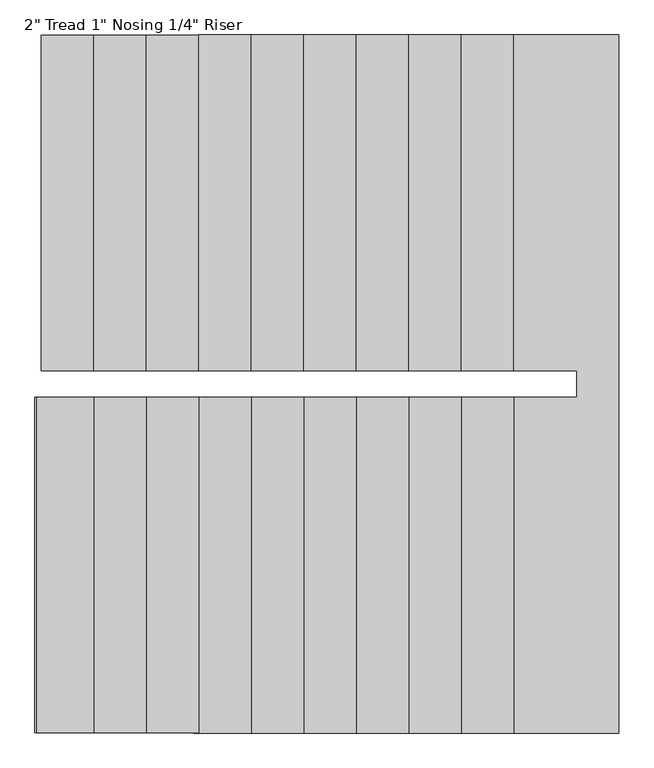
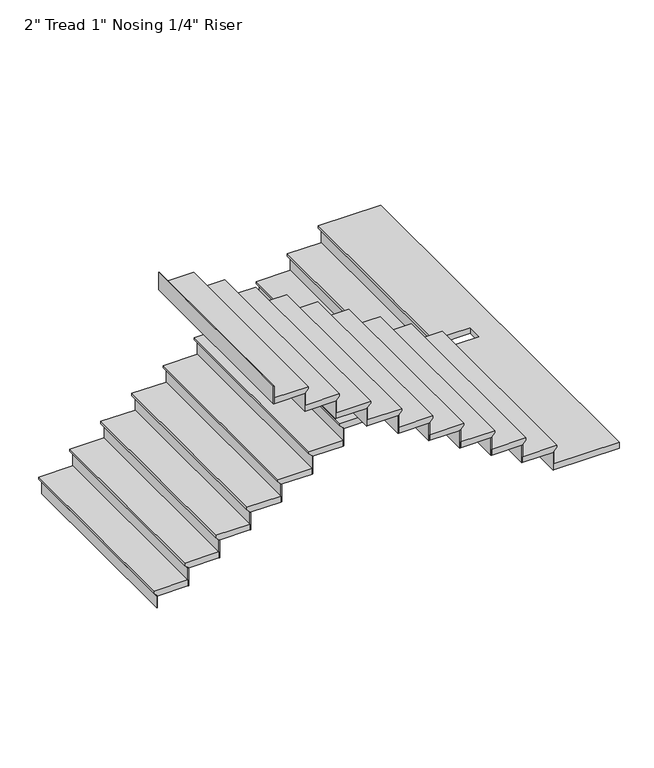
"""IFC4 building model written with IfcOpenShell, lengths in millimetres: stair flight geometry."""

from ifc_helpers import new_model, si_unit, origin, place, context, project, spatial, faceted_brep, source, transform, mapped, element, save


def stair_flight_8d4d0c3c(model_context):
    return source(origin(), model_context, "Body", "Brep", [
        faceted_brep([(-6414.1711241, 10106.9344295, 6229.35), (-6414.1711241, 10106.9344295, 6248.4), (-6414.1711241, 11732.5344295, 6248.4), (-6414.1711241, 11732.5344295, 6229.35), (-6388.7711241, 10106.9344295, 6203.95), (-6388.7711241, 11732.5344295, 6203.95), (-6134.7711241, 10106.9344295, 6248.4), (-6134.7711241, 11732.5344295, 6248.4), (-6388.7711241, 11732.5344295, 6197.6), (-6134.7711241, 11732.5344295, 6197.6), (-6134.7711241, 10106.9344295, 6197.6), (-6388.7711241, 10106.9344295, 6197.6)], [[[0, 1, 2, 3]], [[4, 0, 3, 5]], [[2, 1, 6, 7]], [[8, 9, 10, 11]], [[2, 7, 9, 8, 5, 3]], [[8, 11, 4, 5]], [[6, 1, 0, 4, 11, 10]], [[7, 6, 10, 9]]]),
        faceted_brep([(-6388.7711241, 10106.9344295, 6197.6), (-6388.7711241, 10106.9344295, 6096.0), (-6382.4211241, 10106.9344295, 6096.0), (-6382.4211241, 10106.9344295, 6197.6), (-6388.7711241, 11732.5344295, 6197.6), (-6382.4211241, 11732.5344295, 6197.6), (-6382.4211241, 11732.5344295, 6096.0), (-6388.7711241, 11732.5344295, 6096.0)], [[[0, 1, 2, 3]], [[4, 5, 6, 7]], [[1, 0, 4, 7]], [[2, 1, 7, 6]], [[3, 2, 6, 5]], [[0, 3, 5, 4]]]),
        faceted_brep([(-6134.7711241, 10106.9344295, 6350.0), (-6134.7711241, 10106.9344295, 6197.6), (-6128.4211241, 10106.9344295, 6197.6), (-6128.4211241, 10106.9344295, 6350.0), (-6134.7711241, 11732.5344295, 6350.0), (-6128.4211241, 11732.5344295, 6350.0), (-6128.4211241, 11732.5344295, 6197.6), (-6134.7711241, 11732.5344295, 6197.6)], [[[0, 1, 2, 3]], [[4, 5, 6, 7]], [[1, 0, 4, 7]], [[2, 1, 7, 6]], [[3, 2, 6, 5]], [[0, 3, 5, 4]]]),
        faceted_brep([(-6160.1711241, 11732.5344295, 6400.8), (-6160.1711241, 10106.9344295, 6400.8), (-5880.7711241, 10106.9344295, 6400.8), (-5880.7711241, 11732.5344295, 6400.8), (-6134.7711241, 11732.5344295, 6350.0), (-5880.7711241, 11732.5344295, 6350.0), (-5880.7711241, 10106.9344295, 6350.0), (-6134.7711241, 10106.9344295, 6350.0), (-6134.7711241, 11732.5344295, 6356.35), (-6160.1711241, 11732.5344295, 6381.75), (-6134.7711241, 10106.9344295, 6356.35), (-6160.1711241, 10106.9344295, 6381.75)], [[[0, 1, 2, 3]], [[4, 5, 6, 7]], [[0, 3, 5, 4, 8, 9]], [[4, 7, 10, 8]], [[2, 1, 11, 10, 7, 6]], [[3, 2, 6, 5]], [[11, 1, 0, 9]], [[10, 11, 9, 8]]]),
        faceted_brep([(-5880.7711241, 10106.9344295, 6502.4), (-5880.7711241, 10106.9344295, 6350.0), (-5874.4211241, 10106.9344295, 6350.0), (-5874.4211241, 10106.9344295, 6502.4), (-5880.7711241, 11732.5344295, 6502.4), (-5874.4211241, 11732.5344295, 6502.4), (-5874.4211241, 11732.5344295, 6350.0), (-5880.7711241, 11732.5344295, 6350.0)], [[[0, 1, 2, 3]], [[4, 5, 6, 7]], [[1, 0, 4, 7]], [[2, 1, 7, 6]], [[3, 2, 6, 5]], [[0, 3, 5, 4]]]),
        faceted_brep([(-5906.1711241, 11732.5344295, 6553.2), (-5906.1711241, 10106.9344295, 6553.2), (-5626.7711241, 10106.9344295, 6553.2), (-5626.7711241, 11732.5344295, 6553.2), (-5880.7711241, 11732.5344295, 6502.4), (-5626.7711241, 11732.5344295, 6502.4), (-5626.7711241, 10106.9344295, 6502.4), (-5880.7711241, 10106.9344295, 6502.4), (-5880.7711241, 11732.5344295, 6508.75), (-5906.1711241, 11732.5344295, 6534.15), (-5880.7711241, 10106.9344295, 6508.75), (-5906.1711241, 10106.9344295, 6534.15)], [[[0, 1, 2, 3]], [[4, 5, 6, 7]], [[0, 3, 5, 4, 8, 9]], [[4, 7, 10, 8]], [[2, 1, 11, 10, 7, 6]], [[3, 2, 6, 5]], [[11, 1, 0, 9]], [[10, 11, 9, 8]]]),
        faceted_brep([(-5626.7711241, 10106.9344295, 6654.8), (-5626.7711241, 10106.9344295, 6502.4), (-5620.4211241, 10106.9344295, 6502.4), (-5620.4211241, 10106.9344295, 6654.8), (-5626.7711241, 11732.5344295, 6654.8), (-5620.4211241, 11732.5344295, 6654.8), (-5620.4211241, 11732.5344295, 6502.4), (-5626.7711241, 11732.5344295, 6502.4)], [[[0, 1, 2, 3]], [[4, 5, 6, 7]], [[1, 0, 4, 7]], [[2, 1, 7, 6]], [[3, 2, 6, 5]], [[0, 3, 5, 4]]]),
        faceted_brep([(-5652.1711241, 11732.5344295, 6705.6), (-5652.1711241, 10106.9344295, 6705.6), (-5372.7711241, 10106.9344295, 6705.6), (-5372.7711241, 11732.5344295, 6705.6), (-5626.7711241, 11732.5344295, 6654.8), (-5372.7711241, 11732.5344295, 6654.8), (-5372.7711241, 10106.9344295, 6654.8), (-5626.7711241, 10106.9344295, 6654.8), (-5626.7711241, 11732.5344295, 6661.15), (-5652.1711241, 11732.5344295, 6686.55), (-5626.7711241, 10106.9344295, 6661.15), (-5652.1711241, 10106.9344295, 6686.55)], [[[0, 1, 2, 3]], [[4, 5, 6, 7]], [[0, 3, 5, 4, 8, 9]], [[4, 7, 10, 8]], [[2, 1, 11, 10, 7, 6]], [[3, 2, 6, 5]], [[11, 1, 0, 9]], [[10, 11, 9, 8]]]),
        faceted_brep([(-5372.7711241, 10106.9344295, 6807.2), (-5372.7711241, 10106.9344295, 6654.8), (-5366.4211241, 10106.9344295, 6654.8), (-5366.4211241, 10106.9344295, 6807.2), (-5372.7711241, 11732.5344295, 6807.2), (-5366.4211241, 11732.5344295, 6807.2), (-5366.4211241, 11732.5344295, 6654.8), (-5372.7711241, 11732.5344295, 6654.8)], [[[0, 1, 2, 3]], [[4, 5, 6, 7]], [[1, 0, 4, 7]], [[2, 1, 7, 6]], [[3, 2, 6, 5]], [[0, 3, 5, 4]]]),
        faceted_brep([(-5398.1711241, 11732.5344295, 6858.0), (-5398.1711241, 10106.9344295, 6858.0), (-5118.7711241, 10106.9344295, 6858.0), (-5118.7711241, 11732.5344295, 6858.0), (-5372.7711241, 11732.5344295, 6807.2), (-5118.7711241, 11732.5344295, 6807.2), (-5118.7711241, 10106.9344295, 6807.2), (-5372.7711241, 10106.9344295, 6807.2), (-5372.7711241, 11732.5344295, 6813.55), (-5398.1711241, 11732.5344295, 6838.95), (-5372.7711241, 10106.9344295, 6813.55), (-5398.1711241, 10106.9344295, 6838.95)], [[[0, 1, 2, 3]], [[4, 5, 6, 7]], [[0, 3, 5, 4, 8, 9]], [[4, 7, 10, 8]], [[2, 1, 11, 10, 7, 6]], [[3, 2, 6, 5]], [[11, 1, 0, 9]], [[10, 11, 9, 8]]]),
        faceted_brep([(-5118.7711241, 10106.9344295, 6959.6), (-5118.7711241, 10106.9344295, 6807.2), (-5112.4211241, 10106.9344295, 6807.2), (-5112.4211241, 10106.9344295, 6959.6), (-5118.7711241, 11732.5344295, 6959.6), (-5112.4211241, 11732.5344295, 6959.6), (-5112.4211241, 11732.5344295, 6807.2), (-5118.7711241, 11732.5344295, 6807.2)], [[[0, 1, 2, 3]], [[4, 5, 6, 7]], [[1, 0, 4, 7]], [[2, 1, 7, 6]], [[3, 2, 6, 5]], [[0, 3, 5, 4]]]),
        faceted_brep([(-5144.1711241, 11732.5344295, 7010.4), (-5144.1711241, 10106.9344295, 7010.4), (-4864.7711241, 10106.9344295, 7010.4), (-4864.7711241, 11732.5344295, 7010.4), (-5118.7711241, 11732.5344295, 6959.6), (-4864.7711241, 11732.5344295, 6959.6), (-4864.7711241, 10106.9344295, 6959.6), (-5118.7711241, 10106.9344295, 6959.6), (-5118.7711241, 11732.5344295, 6965.95), (-5144.1711241, 11732.5344295, 6991.35), (-5118.7711241, 10106.9344295, 6965.95), (-5144.1711241, 10106.9344295, 6991.35)], [[[0, 1, 2, 3]], [[4, 5, 6, 7]], [[0, 3, 5, 4, 8, 9]], [[4, 7, 10, 8]], [[2, 1, 11, 10, 7, 6]], [[3, 2, 6, 5]], [[11, 1, 0, 9]], [[10, 11, 9, 8]]]),
        faceted_brep([(-4864.7711241, 10106.9344295, 7112.0), (-4864.7711241, 10106.9344295, 6959.6), (-4858.4211241, 10106.9344295, 6959.6), (-4858.4211241, 10106.9344295, 7112.0), (-4864.7711241, 11732.5344295, 7112.0), (-4858.4211241, 11732.5344295, 7112.0), (-4858.4211241, 11732.5344295, 6959.6), (-4864.7711241, 11732.5344295, 6959.6)], [[[0, 1, 2, 3]], [[4, 5, 6, 7]], [[1, 0, 4, 7]], [[2, 1, 7, 6]], [[3, 2, 6, 5]], [[0, 3, 5, 4]]]),
        faceted_brep([(-4890.1711241, 11732.5344295, 7162.8), (-4890.1711241, 10106.9344295, 7162.8), (-4610.7711241, 10106.9344295, 7162.8), (-4610.7711241, 11732.5344295, 7162.8), (-4864.7711241, 11732.5344295, 7112.0), (-4610.7711241, 11732.5344295, 7112.0), (-4610.7711241, 10106.9344295, 7112.0), (-4864.7711241, 10106.9344295, 7112.0), (-4864.7711241, 11732.5344295, 7118.35), (-4890.1711241, 11732.5344295, 7143.75), (-4864.7711241, 10106.9344295, 7118.35), (-4890.1711241, 10106.9344295, 7143.75)], [[[0, 1, 2, 3]], [[4, 5, 6, 7]], [[0, 3, 5, 4, 8, 9]], [[4, 7, 10, 8]], [[2, 1, 11, 10, 7, 6]], [[3, 2, 6, 5]], [[11, 1, 0, 9]], [[10, 11, 9, 8]]]),
        faceted_brep([(-4610.7711241, 10106.9344295, 7264.4), (-4610.7711241, 10106.9344295, 7112.0), (-4604.4211241, 10106.9344295, 7112.0), (-4604.4211241, 10106.9344295, 7264.4), (-4610.7711241, 11732.5344295, 7264.4), (-4604.4211241, 11732.5344295, 7264.4), (-4604.4211241, 11732.5344295, 7112.0), (-4610.7711241, 11732.5344295, 7112.0)], [[[0, 1, 2, 3]], [[4, 5, 6, 7]], [[1, 0, 4, 7]], [[2, 1, 7, 6]], [[3, 2, 6, 5]], [[0, 3, 5, 4]]]),
        faceted_brep([(-4636.1711241, 11732.5344295, 7315.2), (-4636.1711241, 10106.9344295, 7315.2), (-4356.7711241, 10106.9344295, 7315.2), (-4356.7711241, 11732.5344295, 7315.2), (-4610.7711241, 11732.5344295, 7264.4), (-4356.7711241, 11732.5344295, 7264.4), (-4356.7711241, 10106.9344295, 7264.4), (-4610.7711241, 10106.9344295, 7264.4), (-4610.7711241, 11732.5344295, 7270.75), (-4636.1711241, 11732.5344295, 7296.15), (-4610.7711241, 10106.9344295, 7270.75), (-4636.1711241, 10106.9344295, 7296.15)], [[[0, 1, 2, 3]], [[4, 5, 6, 7]], [[0, 3, 5, 4, 8, 9]], [[4, 7, 10, 8]], [[2, 1, 11, 10, 7, 6]], [[3, 2, 6, 5]], [[11, 1, 0, 9]], [[10, 11, 9, 8]]]),
        faceted_brep([(-4356.7711241, 10106.9344295, 7416.8), (-4356.7711241, 10106.9344295, 7264.4), (-4350.4211241, 10106.9344295, 7264.4), (-4350.4211241, 10106.9344295, 7416.8), (-4356.7711241, 11732.5344295, 7416.8), (-4350.4211241, 11732.5344295, 7416.8), (-4350.4211241, 11732.5344295, 7264.4), (-4356.7711241, 11732.5344295, 7264.4)], [[[0, 1, 2, 3]], [[4, 5, 6, 7]], [[1, 0, 4, 7]], [[2, 1, 7, 6]], [[3, 2, 6, 5]], [[0, 3, 5, 4]]]),
        faceted_brep([(-4382.1711241, 11732.5344295, 7467.6), (-4382.1711241, 10106.9344295, 7467.6), (-4102.7711241, 10106.9344295, 7467.6), (-4102.7711241, 11732.5344295, 7467.6), (-4356.7711241, 11732.5344295, 7416.8), (-4102.7711241, 11732.5344295, 7416.8), (-4102.7711241, 10106.9344295, 7416.8), (-4356.7711241, 10106.9344295, 7416.8), (-4356.7711241, 11732.5344295, 7423.15), (-4382.1711241, 11732.5344295, 7448.55), (-4356.7711241, 10106.9344295, 7423.15), (-4382.1711241, 10106.9344295, 7448.55)], [[[0, 1, 2, 3]], [[4, 5, 6, 7]], [[0, 3, 5, 4, 8, 9]], [[4, 7, 10, 8]], [[2, 1, 11, 10, 7, 6]], [[3, 2, 6, 5]], [[11, 1, 0, 9]], [[10, 11, 9, 8]]]),
        faceted_brep([(-4102.7711241, 10106.9344295, 7569.2), (-4102.7711241, 10106.9344295, 7416.8), (-4096.4211241, 10106.9344295, 7416.8), (-4096.4211241, 10106.9344295, 7569.2), (-4102.7711241, 11732.5344295, 7569.2), (-4096.4211241, 11732.5344295, 7569.2), (-4096.4211241, 11732.5344295, 7416.8), (-4102.7711241, 11732.5344295, 7416.8)], [[[0, 1, 2, 3]], [[4, 5, 6, 7]], [[1, 0, 4, 7]], [[2, 1, 7, 6]], [[3, 2, 6, 5]], [[0, 3, 5, 4]]]),
        faceted_brep([(-4153.5711241, 8354.3344295, 7620.0), (-3620.1711241, 8354.3344295, 7620.0), (-3620.1711241, 11732.5344295, 7620.0), (-4128.1711241, 11732.5344295, 7620.0), (-4128.1711241, 10106.9344295, 7620.0), (-3823.3711241, 10106.9344295, 7620.0), (-3823.3711241, 9979.9344295, 7620.0), (-4153.5711241, 9979.9344295, 7620.0), (-3620.1711241, 8354.3344295, 7569.2), (-4153.5711241, 8354.3344295, 7569.2), (-4153.5711241, 9979.9344295, 7569.2), (-3823.3711241, 9979.9344295, 7569.2), (-3823.3711241, 10106.9344295, 7569.2), (-4102.7711241, 10106.9344295, 7569.2), (-4102.7711241, 11732.5344295, 7569.2), (-3620.1711241, 11732.5344295, 7569.2), (-4102.7711241, 11732.5344295, 7575.55), (-4128.1711241, 11732.5344295, 7600.95), (-4102.7711241, 10106.9344295, 7575.55), (-4128.1711241, 10106.9344295, 7600.95)], [[[0, 1, 2, 3, 4, 5, 6, 7]], [[8, 9, 10, 11, 12, 13, 14, 15]], [[1, 0, 9, 8]], [[2, 1, 8, 15]], [[3, 2, 15, 14, 16, 17]], [[14, 13, 18, 16]], [[5, 4, 19, 18, 13, 12]], [[6, 5, 12, 11]], [[7, 6, 11, 10]], [[0, 7, 10, 9]], [[19, 4, 3, 17]], [[18, 19, 17, 16]]]),
        faceted_brep([(-4153.5711241, 9979.9344295, 7721.6), (-4153.5711241, 9979.9344295, 7569.2), (-4159.9211241, 9979.9344295, 7569.2), (-4159.9211241, 9979.9344295, 7721.6), (-4153.5711241, 8354.3344295, 7721.6), (-4159.9211241, 8354.3344295, 7721.6), (-4159.9211241, 8354.3344295, 7569.2), (-4153.5711241, 8354.3344295, 7569.2)], [[[0, 1, 2, 3]], [[4, 5, 6, 7]], [[1, 0, 4, 7]], [[2, 1, 7, 6]], [[3, 2, 6, 5]], [[0, 3, 5, 4]]]),
        faceted_brep([(-4128.1711241, 8354.3344295, 7772.4), (-4128.1711241, 9979.9344295, 7772.4), (-4407.5711241, 9979.9344295, 7772.4), (-4407.5711241, 8354.3344295, 7772.4), (-4153.5711241, 8354.3344295, 7721.6), (-4407.5711241, 8354.3344295, 7721.6), (-4407.5711241, 9979.9344295, 7721.6), (-4153.5711241, 9979.9344295, 7721.6), (-4153.5711241, 8354.3344295, 7727.95), (-4128.1711241, 8354.3344295, 7753.35), (-4153.5711241, 9979.9344295, 7727.95), (-4128.1711241, 9979.9344295, 7753.35)], [[[0, 1, 2, 3]], [[4, 5, 6, 7]], [[0, 3, 5, 4, 8, 9]], [[4, 7, 10, 8]], [[2, 1, 11, 10, 7, 6]], [[3, 2, 6, 5]], [[11, 1, 0, 9]], [[10, 11, 9, 8]]]),
        faceted_brep([(-4407.5711241, 9979.9344295, 7874.0), (-4407.5711241, 9979.9344295, 7721.6), (-4413.9211241, 9979.9344295, 7721.6), (-4413.9211241, 9979.9344295, 7874.0), (-4407.5711241, 8354.3344295, 7874.0), (-4413.9211241, 8354.3344295, 7874.0), (-4413.9211241, 8354.3344295, 7721.6), (-4407.5711241, 8354.3344295, 7721.6)], [[[0, 1, 2, 3]], [[4, 5, 6, 7]], [[1, 0, 4, 7]], [[2, 1, 7, 6]], [[3, 2, 6, 5]], [[0, 3, 5, 4]]]),
        faceted_brep([(-4382.1711241, 8354.3344295, 7924.8), (-4382.1711241, 9979.9344295, 7924.8), (-4661.5711241, 9979.9344295, 7924.8), (-4661.5711241, 8354.3344295, 7924.8), (-4407.5711241, 8354.3344295, 7874.0), (-4661.5711241, 8354.3344295, 7874.0), (-4661.5711241, 9979.9344295, 7874.0), (-4407.5711241, 9979.9344295, 7874.0), (-4407.5711241, 8354.3344295, 7880.35), (-4382.1711241, 8354.3344295, 7905.75), (-4407.5711241, 9979.9344295, 7880.35), (-4382.1711241, 9979.9344295, 7905.75)], [[[0, 1, 2, 3]], [[4, 5, 6, 7]], [[0, 3, 5, 4, 8, 9]], [[4, 7, 10, 8]], [[2, 1, 11, 10, 7, 6]], [[3, 2, 6, 5]], [[11, 1, 0, 9]], [[10, 11, 9, 8]]]),
        faceted_brep([(-4661.5711241, 9979.9344295, 8026.4), (-4661.5711241, 9979.9344295, 7874.0), (-4667.9211241, 9979.9344295, 7874.0), (-4667.9211241, 9979.9344295, 8026.4), (-4661.5711241, 8354.3344295, 8026.4), (-4667.9211241, 8354.3344295, 8026.4), (-4667.9211241, 8354.3344295, 7874.0), (-4661.5711241, 8354.3344295, 7874.0)], [[[0, 1, 2, 3]], [[4, 5, 6, 7]], [[1, 0, 4, 7]], [[2, 1, 7, 6]], [[3, 2, 6, 5]], [[0, 3, 5, 4]]]),
        faceted_brep([(-4636.1711241, 8354.3344295, 8077.2), (-4636.1711241, 9979.9344295, 8077.2), (-4915.5711241, 9979.9344295, 8077.2), (-4915.5711241, 8354.3344295, 8077.2), (-4661.5711241, 8354.3344295, 8026.4), (-4915.5711241, 8354.3344295, 8026.4), (-4915.5711241, 9979.9344295, 8026.4), (-4661.5711241, 9979.9344295, 8026.4), (-4661.5711241, 8354.3344295, 8032.75), (-4636.1711241, 8354.3344295, 8058.15), (-4661.5711241, 9979.9344295, 8032.75), (-4636.1711241, 9979.9344295, 8058.15)], [[[0, 1, 2, 3]], [[4, 5, 6, 7]], [[0, 3, 5, 4, 8, 9]], [[4, 7, 10, 8]], [[2, 1, 11, 10, 7, 6]], [[3, 2, 6, 5]], [[11, 1, 0, 9]], [[10, 11, 9, 8]]]),
        faceted_brep([(-4915.5711241, 9979.9344295, 8178.8), (-4915.5711241, 9979.9344295, 8026.4), (-4921.9211241, 9979.9344295, 8026.4), (-4921.9211241, 9979.9344295, 8178.8), (-4915.5711241, 8354.3344295, 8178.8), (-4921.9211241, 8354.3344295, 8178.8), (-4921.9211241, 8354.3344295, 8026.4), (-4915.5711241, 8354.3344295, 8026.4)], [[[0, 1, 2, 3]], [[4, 5, 6, 7]], [[1, 0, 4, 7]], [[2, 1, 7, 6]], [[3, 2, 6, 5]], [[0, 3, 5, 4]]]),
        faceted_brep([(-4890.1711241, 8354.3344295, 8229.6), (-4890.1711241, 9979.9344295, 8229.6), (-5169.5711241, 9979.9344295, 8229.6), (-5169.5711241, 8354.3344295, 8229.6), (-4915.5711241, 8354.3344295, 8178.8), (-5169.5711241, 8354.3344295, 8178.8), (-5169.5711241, 9979.9344295, 8178.8), (-4915.5711241, 9979.9344295, 8178.8), (-4915.5711241, 8354.3344295, 8185.15), (-4890.1711241, 8354.3344295, 8210.55), (-4915.5711241, 9979.9344295, 8185.15), (-4890.1711241, 9979.9344295, 8210.55)], [[[0, 1, 2, 3]], [[4, 5, 6, 7]], [[0, 3, 5, 4, 8, 9]], [[4, 7, 10, 8]], [[2, 1, 11, 10, 7, 6]], [[3, 2, 6, 5]], [[11, 1, 0, 9]], [[10, 11, 9, 8]]]),
        faceted_brep([(-5169.5711241, 9979.9344295, 8331.2), (-5169.5711241, 9979.9344295, 8178.8), (-5175.9211241, 9979.9344295, 8178.8), (-5175.9211241, 9979.9344295, 8331.2), (-5169.5711241, 8354.3344295, 8331.2), (-5175.9211241, 8354.3344295, 8331.2), (-5175.9211241, 8354.3344295, 8178.8), (-5169.5711241, 8354.3344295, 8178.8)], [[[0, 1, 2, 3]], [[4, 5, 6, 7]], [[1, 0, 4, 7]], [[2, 1, 7, 6]], [[3, 2, 6, 5]], [[0, 3, 5, 4]]]),
        faceted_brep([(-5144.1711241, 8354.3344295, 8382.0), (-5144.1711241, 9979.9344295, 8382.0), (-5423.5711241, 9979.9344295, 8382.0), (-5423.5711241, 8354.3344295, 8382.0), (-5169.5711241, 8354.3344295, 8331.2), (-5423.5711241, 8354.3344295, 8331.2), (-5423.5711241, 9979.9344295, 8331.2), (-5169.5711241, 9979.9344295, 8331.2), (-5169.5711241, 8354.3344295, 8337.55), (-5144.1711241, 8354.3344295, 8362.95), (-5169.5711241, 9979.9344295, 8337.55), (-5144.1711241, 9979.9344295, 8362.95)], [[[0, 1, 2, 3]], [[4, 5, 6, 7]], [[0, 3, 5, 4, 8, 9]], [[4, 7, 10, 8]], [[2, 1, 11, 10, 7, 6]], [[3, 2, 6, 5]], [[11, 1, 0, 9]], [[10, 11, 9, 8]]]),
        faceted_brep([(-5423.5711241, 9979.9344295, 8483.6), (-5423.5711241, 9979.9344295, 8331.2), (-5429.9211241, 9979.9344295, 8331.2), (-5429.9211241, 9979.9344295, 8483.6), (-5423.5711241, 8354.3344295, 8483.6), (-5429.9211241, 8354.3344295, 8483.6), (-5429.9211241, 8354.3344295, 8331.2), (-5423.5711241, 8354.3344295, 8331.2)], [[[0, 1, 2, 3]], [[4, 5, 6, 7]], [[1, 0, 4, 7]], [[2, 1, 7, 6]], [[3, 2, 6, 5]], [[0, 3, 5, 4]]]),
        faceted_brep([(-5398.1711241, 8354.3344295, 8534.4), (-5398.1711241, 9979.9344295, 8534.4), (-5677.5711241, 9979.9344295, 8534.4), (-5677.5711241, 8354.3344295, 8534.4), (-5423.5711241, 8354.3344295, 8483.6), (-5677.5711241, 8354.3344295, 8483.6), (-5677.5711241, 9979.9344295, 8483.6), (-5423.5711241, 9979.9344295, 8483.6), (-5423.5711241, 8354.3344295, 8489.95), (-5398.1711241, 8354.3344295, 8515.35), (-5423.5711241, 9979.9344295, 8489.95), (-5398.1711241, 9979.9344295, 8515.35)], [[[0, 1, 2, 3]], [[4, 5, 6, 7]], [[0, 3, 5, 4, 8, 9]], [[4, 7, 10, 8]], [[2, 1, 11, 10, 7, 6]], [[3, 2, 6, 5]], [[11, 1, 0, 9]], [[10, 11, 9, 8]]]),
        faceted_brep([(-5677.5711241, 9979.9344295, 8636.0), (-5677.5711241, 9979.9344295, 8483.6), (-5683.9211241, 9979.9344295, 8483.6), (-5683.9211241, 9979.9344295, 8636.0), (-5677.5711241, 8354.3344295, 8636.0), (-5683.9211241, 8354.3344295, 8636.0), (-5683.9211241, 8354.3344295, 8483.6), (-5677.5711241, 8354.3344295, 8483.6)], [[[0, 1, 2, 3]], [[4, 5, 6, 7]], [[1, 0, 4, 7]], [[2, 1, 7, 6]], [[3, 2, 6, 5]], [[0, 3, 5, 4]]]),
        faceted_brep([(-5652.1711241, 8354.3344295, 8686.8), (-5652.1711241, 9979.9344295, 8686.8), (-5931.5711241, 9979.9344295, 8686.8), (-5931.5711241, 8354.3344295, 8686.8), (-5677.5711241, 8354.3344295, 8636.0), (-5931.5711241, 8354.3344295, 8636.0), (-5931.5711241, 9979.9344295, 8636.0), (-5677.5711241, 9979.9344295, 8636.0), (-5677.5711241, 8354.3344295, 8642.35), (-5652.1711241, 8354.3344295, 8667.75), (-5677.5711241, 9979.9344295, 8642.35), (-5652.1711241, 9979.9344295, 8667.75)], [[[0, 1, 2, 3]], [[4, 5, 6, 7]], [[0, 3, 5, 4, 8, 9]], [[4, 7, 10, 8]], [[2, 1, 11, 10, 7, 6]], [[3, 2, 6, 5]], [[11, 1, 0, 9]], [[10, 11, 9, 8]]]),
        faceted_brep([(-5931.5711241, 9979.9344295, 8788.4), (-5931.5711241, 9979.9344295, 8636.0), (-5937.9211241, 9979.9344295, 8636.0), (-5937.9211241, 9979.9344295, 8788.4), (-5931.5711241, 8354.3344295, 8788.4), (-5937.9211241, 8354.3344295, 8788.4), (-5937.9211241, 8354.3344295, 8636.0), (-5931.5711241, 8354.3344295, 8636.0)], [[[0, 1, 2, 3]], [[4, 5, 6, 7]], [[1, 0, 4, 7]], [[2, 1, 7, 6]], [[3, 2, 6, 5]], [[0, 3, 5, 4]]]),
        faceted_brep([(-5906.1711241, 8354.3344295, 8839.2), (-5906.1711241, 9979.9344295, 8839.2), (-6185.5711241, 9979.9344295, 8839.2), (-6185.5711241, 8354.3344295, 8839.2), (-5931.5711241, 8354.3344295, 8788.4), (-6185.5711241, 8354.3344295, 8788.4), (-6185.5711241, 9979.9344295, 8788.4), (-5931.5711241, 9979.9344295, 8788.4), (-5931.5711241, 8354.3344295, 8794.75), (-5906.1711241, 8354.3344295, 8820.15), (-5931.5711241, 9979.9344295, 8794.75), (-5906.1711241, 9979.9344295, 8820.15)], [[[0, 1, 2, 3]], [[4, 5, 6, 7]], [[0, 3, 5, 4, 8, 9]], [[4, 7, 10, 8]], [[2, 1, 11, 10, 7, 6]], [[3, 2, 6, 5]], [[11, 1, 0, 9]], [[10, 11, 9, 8]]]),
        faceted_brep([(-6185.5711241, 9979.9344295, 8940.8), (-6185.5711241, 9979.9344295, 8788.4), (-6191.9211241, 9979.9344295, 8788.4), (-6191.9211241, 9979.9344295, 8940.8), (-6185.5711241, 8354.3344295, 8940.8), (-6191.9211241, 8354.3344295, 8940.8), (-6191.9211241, 8354.3344295, 8788.4), (-6185.5711241, 8354.3344295, 8788.4)], [[[0, 1, 2, 3]], [[4, 5, 6, 7]], [[1, 0, 4, 7]], [[2, 1, 7, 6]], [[3, 2, 6, 5]], [[0, 3, 5, 4]]]),
        faceted_brep([(-6439.5711241, 9979.9344295, 9093.2), (-6439.5711241, 9979.9344295, 8940.8), (-6445.9211241, 9979.9344295, 8940.8), (-6445.9211241, 9979.9344295, 9093.2), (-6439.5711241, 8354.3344295, 9093.2), (-6445.9211241, 8354.3344295, 9093.2), (-6445.9211241, 8354.3344295, 8940.8), (-6439.5711241, 8354.3344295, 8940.8)], [[[0, 1, 2, 3]], [[4, 5, 6, 7]], [[1, 0, 4, 7]], [[2, 1, 7, 6]], [[3, 2, 6, 5]], [[0, 3, 5, 4]]]),
        faceted_brep([(-6160.1711241, 8354.3344295, 8991.6), (-6160.1711241, 9979.9344295, 8991.6), (-6439.5711241, 9979.9344295, 8991.6), (-6439.5711241, 8354.3344295, 8991.6), (-6185.5711241, 8354.3344295, 8940.8), (-6439.5711241, 8354.3344295, 8940.8), (-6439.5711241, 9979.9344295, 8940.8), (-6185.5711241, 9979.9344295, 8940.8), (-6185.5711241, 8354.3344295, 8947.15), (-6160.1711241, 8354.3344295, 8972.55), (-6185.5711241, 9979.9344295, 8947.15), (-6160.1711241, 9979.9344295, 8972.55)], [[[0, 1, 2, 3]], [[4, 5, 6, 7]], [[0, 3, 5, 4, 8, 9]], [[4, 7, 10, 8]], [[2, 1, 11, 10, 7, 6]], [[3, 2, 6, 5]], [[11, 1, 0, 9]], [[10, 11, 9, 8]]]),
    ])


if __name__ == "__main__":
    model = new_model("IFC4")
    model_context = context("Model", 3, world=origin())
    ifc_project = project(units=[si_unit("LENGTHUNIT", "METRE", prefix="MILLI")], contexts=[model_context])
    site = spatial("IfcSite", under=ifc_project)
    building = spatial("IfcBuilding", under=site)
    placement = place(None, origin())
    stair_flight_shape = stair_flight_8d4d0c3c(model_context)
    element("IfcStairFlight", 1, ObjectType="2\" Tread 1\" Nosing 1/4\" Riser", at=placement, inside=building, context=model_context, shape_type="MappedRepresentation", body=[
        mapped(stair_flight_shape, transform((0.0, 0.0, 0.0), x_axis=(1.0, 0.0, 0.0), y_axis=(0.0, 1.0, 0.0), z_axis=(0.0, 0.0, 1.0))),
    ])
    save(model, "model.ifc")
